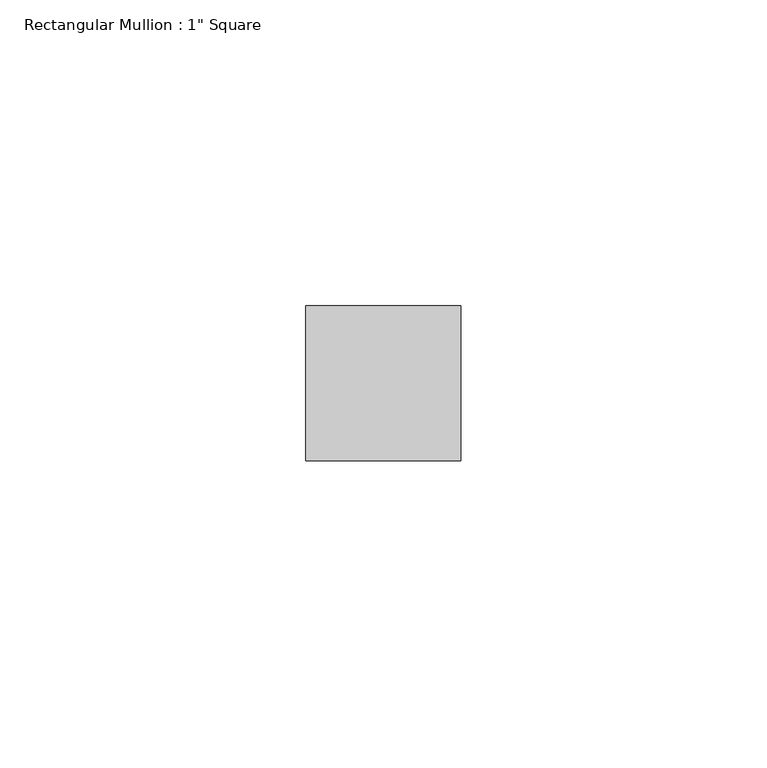
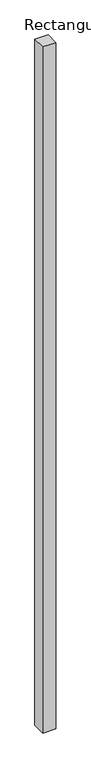
"""IFC4 building model written with IfcOpenShell, lengths in millimetres: member geometry."""

from ifc_helpers import new_model, si_unit, frame, origin, place, context, project, spatial, polyline, outline, extrude, source, transform, mapped, element, save


def member_408d7f8b(model_context):
    return source(origin(), model_context, "Body", "SweptSolid", [
        extrude(outline(polyline([(0.0, 12.7), (0.0, -12.7), (-25.4, -12.7), (-25.4, 12.7), (0.0, 12.7)])), frame((0.0, 0.0, -1384.3), z_axis=(0.0, 0.0, 1.0), x_axis=(1.0, 0.0, 0.0)), (0.0, 0.0, 1.0), 1384.3),
    ])


if __name__ == "__main__":
    model = new_model("IFC4")
    model_context = context("Model", 3, world=origin())
    ifc_project = project(units=[si_unit("LENGTHUNIT", "METRE", prefix="MILLI")], contexts=[model_context])
    site = spatial("IfcSite", under=ifc_project)
    building = spatial("IfcBuilding", under=site)
    placement = place(None, origin())
    member_shape = member_408d7f8b(model_context)
    element("IfcMember", 1, ObjectType="Rectangular Mullion : 1\" Square", at=placement, inside=building, context=model_context, shape_type="MappedRepresentation", body=[
        mapped(member_shape, transform((0.0, 0.0, 0.0), x_axis=(1.0, 0.0, 0.0), y_axis=(0.0, 1.0, 0.0), z_axis=(0.0, 0.0, 1.0))),
    ])
    save(model, "model.ifc")

# Revit data of these elements
# Type "Rectangular Mullion : 1\" Square"
#   built-in parameter 1007304 = 0.0833333 (stored number, unit not read)
#   built-in parameter 1007301 = 0.0416667 (stored number, unit not read)
#   built-in parameter 1007300 = 0.0416667 (stored number, unit not read)
